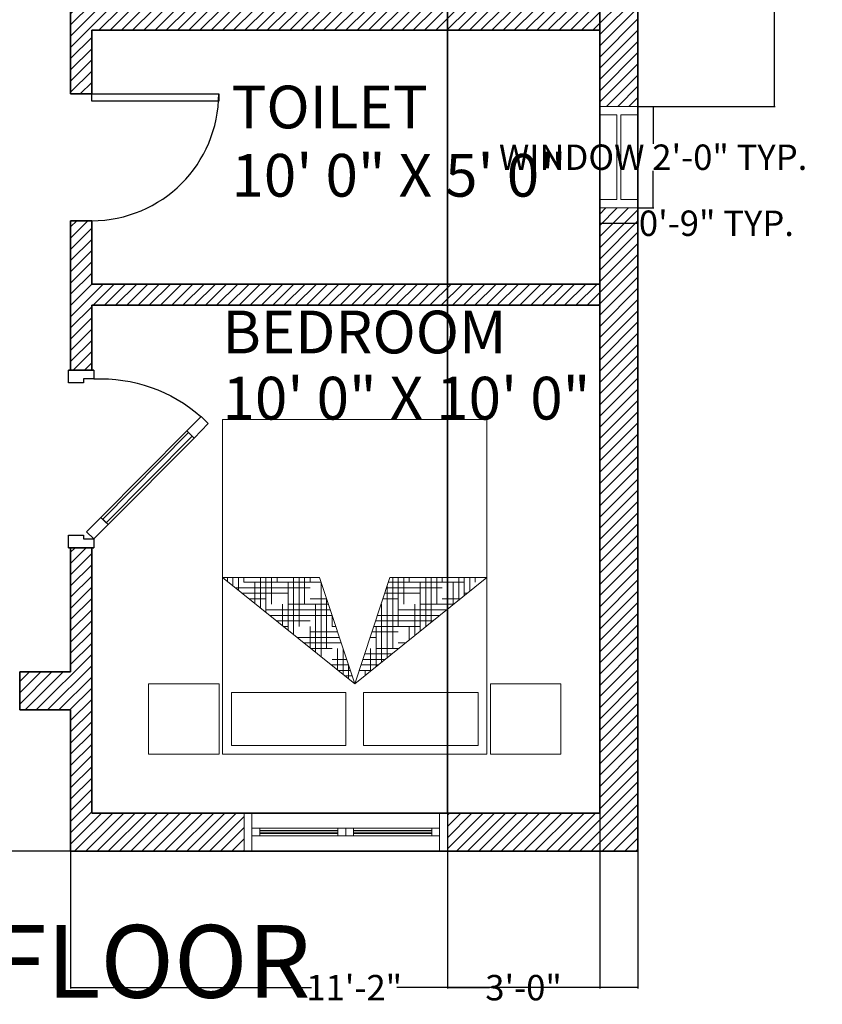
# Model space of a CAD drawing. Units: inches. Extents: x 585 to 1401, y -184 to 463.
# Tile 2 of 8: x 796 to 985, y -179 to 53. Entities that reach past the tile are written whole.
import ezdxf

# ---------------------------------------------------------------- set-up
doc = ezdxf.new("R2010")
doc.units = ezdxf.units.IN
doc.header["$MEASUREMENT"] = 0
for name, color, linetype, lineweight in [('A-ANNO-DIMS', 2, 'Continuous', 18), ('A-ANNO-TEXT', 7, 'Continuous', 25), ('A-AREA-IDEN', 7, 'Continuous', 18), ('A-Door', 150, 'Continuous', 25), ('A-FURN', 8, 'Continuous', 18), ('A-Glaz', 140, 'Continuous', 18), ('A-Wall', 7, 'Continuous', 35), ('A-WALL-PATT', 252, 'Continuous', 13)]:
    doc.layers.add(name, color=color, linetype=linetype, lineweight=lineweight)
doc.styles.get("Standard").update_dxf_attribs({"font": 'arial.ttf'})
doc.dimstyles.get("Standard").update_dxf_attribs({"dimtxt": 6, "dimasz": 0.18, "dimexe": 0.18, "dimexo": 0.0625, "dimgap": 0.09, "dimtad": 0, "dimtih": 1, "dimtoh": 1, "dimdec": 0, "dimzin": 0, "dimdsep": 46, "dimlunit": 3, "dimtxsty": 'Standard', "dimblk": 'ARCHTICK', "dimcen": 0.09, "dimadec": 0, "dimazin": 0, "dimtfac": 1, "dimtdec": 0, "dimtofl": 0, "dimtmove": 0, "dimatfit": 3, "dimfxl": 1, "dimtolj": 1, "dimtzin": 0, "dimarcsym": 0})

# ---------------------------------------------------------------- blocks, each defined once
blk = doc.blocks.new('*U9')
for p, q in [((0, 0), (0, -5)), ((30, 0), (30, -5))]:
    blk.add_line(p, q)
blk.add_lwpolyline([(0, 0), (0, 30), (1.75, 30), (1.75, 0)], close=True)
blk.add_arc((0, 0), 30, 0, 90)
blk = doc.blocks.new('A$C1DF4181C')
blk.add_lwpolyline([(120, 128), (460.7, 466.1), (432.5, 494.5), (91.8, 156.4)], close=True)
blk.add_arc((72.4, 128.7), 593.3, 357.2313, 41.4937)
at = {"layer": 'A-Door'}
for points in [[(517.5, 522.4), (460.7, 466.1), (432.5, 494.5), (489.3, 550.8)], [(63.2, 71.6), (120, 128), (91.8, 156.4), (35, 100)], [(35, 100), (0, 100), (0, 0), (50, 0), (50, 50), (50, 60), (35, 60)], [(665, 100), (665, 60), (650, 60), (650, 50), (650, 0), (700, 0), (700, 100)]]:
    blk.add_lwpolyline(points, close=True, dxfattribs=at)
at = {"layer": 'A-Glaz'}
blk.add_lwpolyline([(112.9, 135.1), (453.6, 473.2), (439.5, 487.4), (98.8, 149.3)], close=True, dxfattribs=at)
at = {"layer": 'A-Wall'}
for p, q in [((0, 0), (0, 100)), ((0, 100), (0, 0)), ((700, 0), (700, 100)), ((700, 0), (700, 100))]:
    blk.add_line(p, q, dxfattribs=at)
blk = doc.blocks.new('*X23')
at = {"color": 0}
for p, q in [((20.25, 14.8125), (20.2772, 14.8125)), ((20.1875, 14.75), (20.1875, 14.7669)), ((20.199, 14.7812), (20.2772, 14.7812)), ((20.1487, 14.7188), (20.2772, 14.7188)), ((20.1562, 14.625), (20.1562, 14.7281)), ((20.1739, 14.75), (20.2772, 14.75)), ((20.25, 14.3194), (20.25, 14.75)), ((20.0938, 14.375), (20.0938, 14.6504)), ((20.0984, 14.6562), (20.125, 14.6562)), ((20.1236, 14.6875), (20.25, 14.6875)), ((20.125, 14.5), (20.125, 14.6893)), ((20.0625, 14.2573), (20.0625, 14.6116)), ((20.125, 14.5938), (20.2772, 14.5938)), ((20.2188, 14.3091), (20.2188, 14.625)), ((20.25, 14.625), (20.2772, 14.625)), ((19.9979, 14.5312), (20.2772, 14.5312)), ((20.023, 14.5625), (20.2772, 14.5625)), ((20.0312, 14.2469), (20.0312, 14.5727)), ((19.9727, 14.5), (20.25, 14.5)), ((20, 14.2366), (20, 14.5)), ((20.1875, 14.2987), (20.1875, 14.5)), ((19.9225, 14.4375), (20, 14.4375)), ((19.9476, 14.4688), (20.125, 14.4688)), ((20.25, 14.4375), (20.2772, 14.4375)), ((19.875, 14.25), (19.875, 14.3785)), ((19.9062, 14.375), (19.9062, 14.4174)), ((19.9688, 14.2262), (19.9688, 14.375)), ((20, 14.375), (20.2772, 14.375)), ((20.125, 14.4062), (20.2772, 14.4062)), ((20.1562, 14.2884), (20.1562, 14.375)), ((19.8219, 14.3125), (20.2291, 14.3125)), ((19.8438, 14.1848), (19.8438, 14.3397)), ((19.875, 14.3438), (20.2772, 14.3438)), ((19.7812, 14.1641), (19.7812, 14.262)), ((19.7967, 14.2812), (20.125, 14.2812)), ((19.8125, 14.1744), (19.8125, 14.3008)), ((19.7465, 14.2188), (19.875, 14.2188)), ((19.75, 14.1537), (19.75, 14.2231)), ((19.7716, 14.25), (20, 14.25)), ((19.9375, 14.2159), (19.9375, 14.25)), ((19.7213, 14.1875), (19.75, 14.1875)), ((19.7018, 14.0938), (19.7786, 14.0938)), ((19.7188, 14.0726), (19.7188, 14.1136)), ((19.75, 14.0338), (19.75, 14.1032)), ((19.7812, 13.9949), (19.7812, 14.0929)), ((19.7269, 14.0625), (19.8728, 14.0625)), ((19.752, 14.0312), (19.875, 14.0312)), ((19.8125, 14), (19.8125, 14.0825)), ((19.9062, 13.8396), (19.9062, 14.0514)), ((19.9375, 13.8007), (19.9375, 14.0411)), ((19.9688, 13.875), (19.9688, 14.0307)), ((19.875, 13.8784), (19.875, 14)), ((20, 14), (20, 14.0204)), ((20, 14), (20.0614, 14)), ((20.0625, 13.6454), (20.0625, 13.9996)), ((20.0938, 13.625), (20.0938, 13.9893)), ((20.125, 13.75), (20.125, 13.9789)), ((19.8275, 13.9375), (20.25, 13.9375)), ((19.875, 13.9688), (20.1557, 13.9688)), ((20.1562, 13.875), (20.1562, 13.9686)), ((20.25, 13.5), (20.25, 13.9375)), ((19.8526, 13.9062), (20.125, 13.9062)), ((19.8777, 13.875), (20, 13.875)), ((20.0312, 13.6842), (20.0312, 13.875)), ((20.2188, 13.4511), (20.2188, 13.875)), ((20.25, 13.875), (20.2772, 13.875)), ((20, 13.8125), (20.2772, 13.8125)), ((20.125, 13.8438), (20.2772, 13.8438)), ((19.9532, 13.7812), (20.2772, 13.7812)), ((19.9783, 13.75), (20.25, 13.75)), ((20, 13.723), (20, 13.75)), ((20.1875, 13.49), (20.1875, 13.75)), ((20.0035, 13.7188), (20.125, 13.7188)), ((20.125, 13.6562), (20.2772, 13.6562)), ((20.25, 13.6875), (20.2772, 13.6875)), ((20.0789, 13.625), (20.2772, 13.625)), ((20.104, 13.5938), (20.2772, 13.5938)), ((20.1562, 13.5288), (20.1562, 13.625)), ((20.1292, 13.5625), (20.25, 13.5625)), ((20.25, 13.5), (20.2772, 13.5)), ((20.2046, 13.4688), (20.2772, 13.4688)), ((20.2297, 13.4375), (20.2772, 13.4375)), ((20.2549, 13.4062), (20.2772, 13.4062))]:
    blk.add_line(p, q, dxfattribs=at)
blk = doc.blocks.new('MAT-P02')
for p, q in [((-1.17, 0), (-1.17, -0.4)), ((-1.17, 0), (-0.77, 0)), ((-0.77, 0), (-0.77, -0.4)), ((-0.75, 0), (0.75, 0)), ((-0.75, 0), (-0.75, -1.9)), ((0.75, 0), (0.75, -1.9)), ((0.77, 0), (1.17, 0)), ((0.77, 0), (0.77, -0.4)), ((1.17, 0), (1.17, -0.4)), ((-0.7, -0.05), (-0.7, -0.35)), ((-0.7, -0.05), (-0.05, -0.05)), ((-0.05, -0.35), (-0.05, -0.05)), ((0.05, -0.05), (0.7, -0.05)), ((0.05, -0.35), (0.05, -0.05)), ((0.7, -0.05), (0.7, -0.35)), ((-0.7, -0.35), (-0.05, -0.35)), ((0.05, -0.35), (0.7, -0.35)), ((-1.17, -0.4), (-0.77, -0.4)), ((-0.75, -1.0034), (0, -0.4)), ((0, -0.4), (-0.75, -1.0034)), ((0, -0.4), (-0.2, -1.0034)), ((0, -0.4), (0.2, -1.0034)), ((0, -0.4), (0.75, -1.0034)), ((0.77, -0.4), (1.17, -0.4)), ((-0.75, -1.0034), (-0.2, -1.0034)), ((0.2, -1.0034), (0.75, -1.0034)), ((0.75, -1.9), (-0.75, -1.9))]:
    blk.add_line(p, q)
at = {"xscale": -1, "rotation": 90}
blk.add_blockref('*X23', (14.1285, 19.2738), dxfattribs=at)
blk = doc.blocks.new('WIN-48-DOUBLE-PANEL')
for p, q in [((48, 9), (0, 9)), ((0, 9), (0, 0)), ((1.85, 9), (0, 9)), ((0, 9), (0, 0)), ((1.85, 0), (1.85, 9)), ((1.85, 0), (1.85, 9)), ((46.15, 9), (48, 9)), ((46.15, 0), (46.15, 9)), ((46.15, 0), (46.15, 9)), ((46.15, 0), (46.15, 9)), ((48, 9), (48, 0)), ((48, 0), (48, 9)), ((1.85, 5.44), (46.15, 5.44)), ((3.69, 3.6), (3.69, 5.44)), ((3.69, 4.89), (22.15, 4.89)), ((22.15, 5.44), (22.15, 3.6)), ((24, 5.44), (24, 3.6)), ((25.85, 5.44), (25.85, 3.6)), ((44.31, 4.89), (25.85, 4.89)), ((44.31, 3.6), (44.31, 5.44)), ((1.85, 3.6), (46.15, 3.6)), ((3.69, 4.52), (22.15, 4.52)), ((3.69, 4.15), (22.15, 4.15)), ((44.31, 4.52), (25.85, 4.52)), ((44.31, 4.15), (25.85, 4.15)), ((0, 0), (1.85, 0)), ((48, 0), (0, 0)), ((48, 0), (46.15, 0))]:
    blk.add_line(p, q)
blk = doc.blocks.new('WIN-24-SINGLE-PANEL')
for p, q in [((0, 0), (0, 24)), ((0, 24), (9, 24)), ((9, 24), (9, 0)), ((0, 22), (4, 22)), ((4, 22), (4, 2)), ((5, 22), (9, 22)), ((5, 22), (5, 2)), ((4, 2), (0, 2)), ((9, 0), (0, 0)), ((9, 2), (5, 2))]:
    blk.add_line(p, q)
blk = doc.blocks.new('_ArchTick')
at = {"color": 0, "linetype": 'ByBlock', "const_width": 0.15}
blk.add_lwpolyline([(-0.5, -0.5), (0.5, 0.5)], dxfattribs=at)
blk = doc.blocks.new('*D40')
at = {"layer": 'A-ANNO-DIMS', "color": 0, "lineweight": -2, "transparency": 16777216}
for p, q in [((941.59, 32.77), (945.31, 32.77)), ((945.13, 32.77), (945.13, 23.97)), ((945.13, 8.77), (945.13, 17.58)), ((941.59, 8.77), (945.31, 8.77))]:
    blk.add_line(p, q, dxfattribs=at)
at = {"layer": 'Defpoints', "color": 0, "transparency": 16777216}
for p in [(941.53, 32.77), (945.13, 32.77), (941.53, 8.77)]:
    blk.add_point(p, dxfattribs=at)
at = {"layer": 'A-ANNO-DIMS', "color": 0, "lineweight": -2, "transparency": 16777216, "xscale": 0.18, "yscale": 0.18, "zscale": 0.18}
for p, rotation in [((945.13, 32.77), 90), ((945.13, 8.77), 270)]:
    blk.add_blockref('_ArchTick', p, dxfattribs=dict(at, rotation=rotation))
at = {"layer": 'A-ANNO-DIMS', "color": 0, "transparency": 16777216, "insert": (945.13, 20.77), "char_height": 6, "attachment_point": 5}
blk.add_mtext('\\A1;WINDOW 2\'-0" TYP.', dxfattribs=at)
blk = doc.blocks.new('*D41')
at = {"layer": 'A-ANNO-DIMS', "color": 0, "lineweight": -2, "transparency": 16777216}
for p, q in [((932.53, 8.71), (932.53, 4.99)), ((941.53, 8.71), (941.53, 4.99)), ((932.53, 5.17), (941.53, 5.17)), ((941.53, 5.17), (941.71, 5.17))]:
    blk.add_line(p, q, dxfattribs=at)
at = {"layer": 'Defpoints', "color": 0, "transparency": 16777216}
for p in [(932.53, 8.77), (941.53, 8.77), (941.53, 5.17)]:
    blk.add_point(p, dxfattribs=at)
at = {"layer": 'A-ANNO-DIMS', "color": 0, "lineweight": -2, "transparency": 16777216, "xscale": 0.18, "yscale": 0.18, "zscale": 0.18, "rotation": 180}
blk.add_blockref('_ArchTick', (932.53, 5.17), dxfattribs=at)
at = {"layer": 'A-ANNO-DIMS', "color": 0, "lineweight": -2, "transparency": 16777216, "xscale": 0.18, "yscale": 0.18, "zscale": 0.18}
blk.add_blockref('_ArchTick', (941.53, 5.17), dxfattribs=at)
at = {"layer": 'A-ANNO-DIMS', "color": 0, "transparency": 16777216, "insert": (960.08, 5.17), "char_height": 6, "attachment_point": 5}
blk.add_mtext('\\A1;0\'-9" TYP.', dxfattribs=at)
blk = doc.blocks.new('*D76')
at = {"layer": 'A-ANNO-DIMS', "color": 0, "lineweight": -2, "transparency": 16777216}
for p, q in [((654.47, 422.15), (622.1, 422.15)), ((622.28, 422.15), (622.28, 142.65)), ((622.28, -143.23), (622.28, 136.27)), ((807.47, -143.23), (622.1, -143.23))]:
    blk.add_line(p, q, dxfattribs=at)
at = {"layer": 'Defpoints', "color": 0, "transparency": 16777216}
for p in [(622.28, 422.15), (654.53, 422.15), (807.53, -143.23)]:
    blk.add_point(p, dxfattribs=at)
at = {"layer": 'A-ANNO-DIMS', "color": 0, "lineweight": -2, "transparency": 16777216, "xscale": 0.18, "yscale": 0.18, "zscale": 0.18}
for p, rotation in [((622.28, 422.15), 90), ((622.28, -143.23), 270)]:
    blk.add_blockref('_ArchTick', p, dxfattribs=dict(at, rotation=rotation))
at = {"layer": 'A-ANNO-DIMS', "color": 0, "transparency": 16777216, "insert": (622.28, 139.46), "char_height": 6, "attachment_point": 5}
blk.add_mtext('\\A1;47\'-1 1/2"', dxfattribs=at)
blk = doc.blocks.new('*D77')
at = {"layer": 'A-ANNO-DIMS', "color": 0, "lineweight": -2, "transparency": 16777216}
for p, q in [((807.53, -143.29), (807.53, -175.66)), ((941.53, -143.29), (941.53, -175.66)), ((807.53, -175.48), (864.41, -175.48)), ((941.53, -175.48), (884.64, -175.48))]:
    blk.add_line(p, q, dxfattribs=at)
at = {"layer": 'Defpoints', "color": 0, "transparency": 16777216}
for p in [(807.53, -143.23), (941.53, -143.23), (941.53, -175.48)]:
    blk.add_point(p, dxfattribs=at)
at = {"layer": 'A-ANNO-DIMS', "color": 0, "lineweight": -2, "transparency": 16777216, "xscale": 0.18, "yscale": 0.18, "zscale": 0.18, "rotation": 180}
blk.add_blockref('_ArchTick', (807.53, -175.48), dxfattribs=at)
at = {"layer": 'A-ANNO-DIMS', "color": 0, "lineweight": -2, "transparency": 16777216, "xscale": 0.18, "yscale": 0.18, "zscale": 0.18}
blk.add_blockref('_ArchTick', (941.53, -175.48), dxfattribs=at)
at = {"layer": 'A-ANNO-DIMS', "color": 0, "transparency": 16777216, "insert": (874.53, -175.48), "char_height": 6, "attachment_point": 5}
blk.add_mtext('\\A1;11\'-2"', dxfattribs=at)
blk = doc.blocks.new('*D83')
at = {"layer": 'A-ANNO-DIMS', "color": 0, "lineweight": -2, "transparency": 16777216}
for p, q in [((896.53, 413.09), (896.53, -175.66)), ((932.53, 413.09), (932.53, -175.66)), ((896.53, -175.48), (906.47, -175.48)), ((932.53, -175.48), (922.59, -175.48))]:
    blk.add_line(p, q, dxfattribs=at)
at = {"layer": 'Defpoints', "color": 0, "transparency": 16777216}
for p in [(896.53, 413.15), (932.53, 413.15), (932.53, -175.48)]:
    blk.add_point(p, dxfattribs=at)
at = {"layer": 'A-ANNO-DIMS', "color": 0, "lineweight": -2, "transparency": 16777216, "xscale": 0.18, "yscale": 0.18, "zscale": 0.18, "rotation": 180}
blk.add_blockref('_ArchTick', (896.53, -175.48), dxfattribs=at)
at = {"layer": 'A-ANNO-DIMS', "color": 0, "lineweight": -2, "transparency": 16777216, "xscale": 0.18, "yscale": 0.18, "zscale": 0.18}
blk.add_blockref('_ArchTick', (932.53, -175.48), dxfattribs=at)
at = {"layer": 'A-ANNO-DIMS', "color": 0, "transparency": 16777216, "insert": (914.53, -175.48), "char_height": 6, "attachment_point": 5}
blk.add_mtext('\\A1;3\'-0"', dxfattribs=at)
blk = doc.blocks.new('*D86')
at = {"layer": 'A-ANNO-DIMS', "color": 0, "lineweight": -2, "transparency": 16777216}
for p, q in [((941.59, 91.77), (973.96, 91.77)), ((973.78, 91.77), (973.78, 65.37)), ((973.78, 32.77), (973.78, 59.17)), ((941.59, 32.77), (973.96, 32.77))]:
    blk.add_line(p, q, dxfattribs=at)
at = {"layer": 'Defpoints', "color": 0, "transparency": 16777216}
for p in [(941.53, 91.77), (973.78, 91.77), (941.53, 32.77)]:
    blk.add_point(p, dxfattribs=at)
at = {"layer": 'A-ANNO-DIMS', "color": 0, "lineweight": -2, "transparency": 16777216, "xscale": 0.18, "yscale": 0.18, "zscale": 0.18}
for p, rotation in [((973.78, 91.77), 90), ((973.78, 32.77), 270)]:
    blk.add_blockref('_ArchTick', p, dxfattribs=dict(at, rotation=rotation))
at = {"layer": 'A-ANNO-DIMS', "color": 0, "transparency": 16777216, "insert": (973.78, 62.27), "char_height": 6, "attachment_point": 5}
blk.add_mtext('\\A1;4\'-11"', dxfattribs=at)
blk = doc.blocks.new('*D88')
at = {"layer": 'A-ANNO-DIMS', "color": 0, "lineweight": -2, "transparency": 16777216}
for p, q in [((896.53, -134.17), (896.53, 454.58)), ((896.53, 454.4), (906.47, 454.4)), ((932.53, 454.4), (922.59, 454.4)), ((932.53, -134.17), (932.53, 454.58))]:
    blk.add_line(p, q, dxfattribs=at)
at = {"layer": 'Defpoints', "color": 0, "transparency": 16777216}
for p in [(932.53, 454.4), (896.53, -134.23), (932.53, -134.23)]:
    blk.add_point(p, dxfattribs=at)
at = {"layer": 'A-ANNO-DIMS', "color": 0, "lineweight": -2, "transparency": 16777216, "xscale": 0.18, "yscale": 0.18, "zscale": 0.18, "rotation": 180}
blk.add_blockref('_ArchTick', (896.53, 454.4), dxfattribs=at)
at = {"layer": 'A-ANNO-DIMS', "color": 0, "lineweight": -2, "transparency": 16777216, "xscale": 0.18, "yscale": 0.18, "zscale": 0.18}
blk.add_blockref('_ArchTick', (932.53, 454.4), dxfattribs=at)
at = {"layer": 'A-ANNO-DIMS', "color": 0, "transparency": 16777216, "insert": (914.53, 454.4), "char_height": 6, "attachment_point": 5}
blk.add_mtext('\\A1;3\'-0"', dxfattribs=at)

msp = doc.modelspace()

# ---------------------------------------------------------------- hatches: boundary and pattern name
at = {"layer": 'A-WALL-PATT'}
h = msp.add_hatch(dxfattribs=at)
h.set_pattern_fill('ANSI31', color=256, scale=15)
h.set_pattern_definition([(45, (599.059, -1e-14), (-1.325825, 1.325825), [])])
h.paths.add_polyline_path([(711.53, 422.15), (654.53, 422.15), (654.53, -109.85), (680.03, -109.85), (680.03, -100.85), (663.53, -100.85), (663.53, 48.87), (759.53, 48.87), (759.53, 57.87), (663.53, 57.87), (663.53, 144.15), (663.53, 264.15), (812.53, 264.15), (812.53, 269.15), (663.53, 269.15), (663.53, 413.15), (711.53, 413.15)])
h.paths.add_polyline_path([(753.53, -100.85), (728.03, -100.85), (728.03, -109.85), (753.53, -109.85)], flags=17)
h.paths.add_polyline_path([(812.53, -71.54), (807.53, -71.54), (807.53, -100.85), (795.53, -100.85), (795.53, -109.85), (807.53, -109.85), (807.53, -143.23), (848.53, -143.23), (848.53, -134.23), (812.53, -134.23)])
h.paths.add_polyline_path([(941.53, 8.77), (932.53, 8.77), (932.53, -9.23), (812.53, -9.23), (812.53, 5.77), (807.53, 5.77), (807.53, -29.54), (812.53, -29.54), (812.53, -14.23), (932.53, -14.23), (932.53, -134.23), (896.53, -134.23), (896.53, -143.23), (941.53, -143.23)])
h.paths.add_polyline_path([(941.53, 91.77), (932.53, 91.77), (932.53, 55.77), (812.53, 55.77), (812.53, 98.58), (807.53, 98.58), (807.53, 35.77), (812.53, 35.77), (812.53, 50.77), (932.53, 50.77), (932.53, 32.77), (941.53, 32.77)])
h.paths.add_polyline_path([(941.53, 222.04), (932.53, 222.04), (932.53, 180.77), (807.53, 180.77), (807.53, 140.58), (812.53, 140.58), (812.53, 175.77), (932.53, 175.77), (932.53, 139.77), (941.53, 139.77)])
h.paths.add_polyline_path([(941.53, 422.15), (896.53, 422.15), (896.53, 413.15), (932.53, 413.15), (932.53, 317.15), (896.53, 317.15), (896.53, 312.15), (932.53, 312.15), (932.53, 270.04), (941.53, 270.04)])
h.paths.add_polyline_path([(848.53, 422.15), (759.53, 422.15), (759.53, 413.15), (807.53, 413.15), (807.53, 312.15), (848.53, 312.15), (848.53, 317.15), (812.53, 317.15), (812.53, 413.15), (848.53, 413.15)])

# ---------------------------------------------------------------- linework, layer by layer
at = {"layer": 'A-Wall'}
for p, q in [((941.53, 422.15), (941.53, -143.23)), ((807.53, 98.58), (807.53, 35.77)), ((812.53, 50.77), (932.53, 50.77)), ((812.53, 50.77), (812.53, 35.77)), ((932.53, 50.77), (932.53, -9.23)), ((812.53, 35.77), (807.53, 35.77)), ((812.53, 5.77), (807.53, 5.77)), ((807.53, 5.77), (807.53, -29.54)), ((812.53, 5.77), (812.53, -9.23)), ((812.53, -9.23), (932.53, -9.23)), ((812.53, -14.23), (932.53, -14.23)), ((812.53, -14.23), (812.53, -29.54)), ((932.53, -14.23), (932.53, -134.23)), ((807.53, -29.54), (812.53, -29.54)), ((807.53, -71.54), (812.53, -71.54)), ((807.53, -71.54), (807.53, -100.85)), ((812.53, -71.54), (812.53, -134.23)), ((795.53, -100.85), (795.53, -109.85)), ((795.53, -100.85), (807.53, -100.85)), ((795.53, -109.85), (807.53, -109.85)), ((807.53, -109.85), (807.53, -143.23)), ((812.53, -134.23), (932.53, -134.23)), ((807.53, -143.23), (941.53, -143.23))]:
    msp.add_line(p, q, dxfattribs=at)

# ---------------------------------------------------------------- block references
at = {"layer": 'A-Door', "rotation": 270}
msp.add_blockref('*U9', (812.53, 35.77), dxfattribs=at)
at = {"layer": 'A-Door', "xscale": -0.0599999999683043, "yscale": 0.0599999999683043, "zscale": 0.0599999999683043, "rotation": 270}
msp.add_blockref('A$C1DF4181C', (807.03, -71.54), dxfattribs=at)
at = {"layer": 'A-FURN', "xscale": 41.63451012544946, "yscale": 41.63451012544946, "zscale": 41.63451012544946, "rotation": 180}
msp.add_blockref('MAT-P02', (874.66, -120.33), dxfattribs=at)
at = {"layer": 'A-Glaz'}
for name, p in [('WIN-24-SINGLE-PANEL', (932.53, 8.77)), ('WIN-48-DOUBLE-PANEL', (848.53, -143.23))]:
    msp.add_blockref(name, p, dxfattribs=at)

# ---------------------------------------------------------------- texts
at = {"layer": 'A-ANNO-TEXT'}
msp.add_text('GROUND FLOOR', height=17.1732, dxfattribs=at).set_placement((685.33, -177.86))
at = {"layer": 'A-AREA-IDEN'}
for s, height, p in [('TOILET', 10.101, (845.54, 27.59)), ('10\' 0" X 5\' 0"', 10.1013, (845.54, 11.45)), ('BEDROOM', 10.101, (843.44, -25.59)), ('10\' 0" X 10\' 0"', 10.1013, (843.44, -41.22))]:
    msp.add_text(s, height=height, dxfattribs=at).set_placement(p)

# ---------------------------------------------------------------- dimensions: what is measured, and where the dimension line sits
at = {"layer": 'A-ANNO-DIMS'}
for base, p1, p2, picture, middle in [((932.53, 454.4), (896.53, -134.23), (932.53, -134.23), '*D88', (914.53, 454.4)), ((932.53, -175.48), (896.53, 413.15), (932.53, 413.15), '*D83', (914.53, -175.48)), ((941.53, -175.48), (807.53, -143.23), (941.53, -143.23), '*D77', (874.53, -175.48))]:
    dim = msp.add_linear_dim(base=base, p1=p1, p2=p2, dimstyle='Standard', override={"dimdec": 1, "dimlfac": 1, "dimrnd": 0, "dimzin": 1, "dimdsep": 46, "dimlunit": 4, "dimfrac": 2}, dxfattribs=at)
    dim.commit()
    dim.dimension.update_dxf_attribs({"geometry": picture, "text_midpoint": middle})
for base, p1, p2, picture, middle in [((622.28, 422.15), (807.53, -143.23), (654.53, 422.15), '*D76', (622.28, 139.46)), ((973.78, 91.77), (941.53, 32.77), (941.53, 91.77), '*D86', (973.78, 62.27))]:
    dim = msp.add_linear_dim(base=base, p1=p1, p2=p2, angle=90, dimstyle='Standard', override={"dimdec": 1, "dimlfac": 1, "dimrnd": 0, "dimzin": 1, "dimdsep": 46, "dimlunit": 4, "dimfrac": 2}, dxfattribs=at)
    dim.commit()
    dim.dimension.update_dxf_attribs({"geometry": picture, "text_midpoint": middle})
dim = msp.add_linear_dim(base=(945.13, 32.77), p1=(941.53, 8.77), p2=(941.53, 32.77), angle=90, text='WINDOW <> TYP.', dimstyle='Standard', override={"dimdec": 1, "dimlfac": 1, "dimrnd": 0, "dimzin": 1, "dimdsep": 46, "dimlunit": 4, "dimfrac": 2}, dxfattribs=at)
dim.commit()
dim.dimension.update_dxf_attribs({"geometry": '*D40', "text_midpoint": (945.13, 20.77)})
dim = msp.add_linear_dim(base=(941.53, 5.17), p1=(932.53, 8.77), p2=(941.53, 8.77), text='<> TYP.', dimstyle='Standard', override={"dimdec": 1, "dimlfac": 1, "dimrnd": 0, "dimzin": 1, "dimdsep": 46, "dimlunit": 4, "dimfrac": 2}, dxfattribs=at)
dim.commit()
dim.dimension.update_dxf_attribs({"geometry": '*D41', "text_midpoint": (960.08, 5.17)})

doc.saveas('drawing.dxf')
